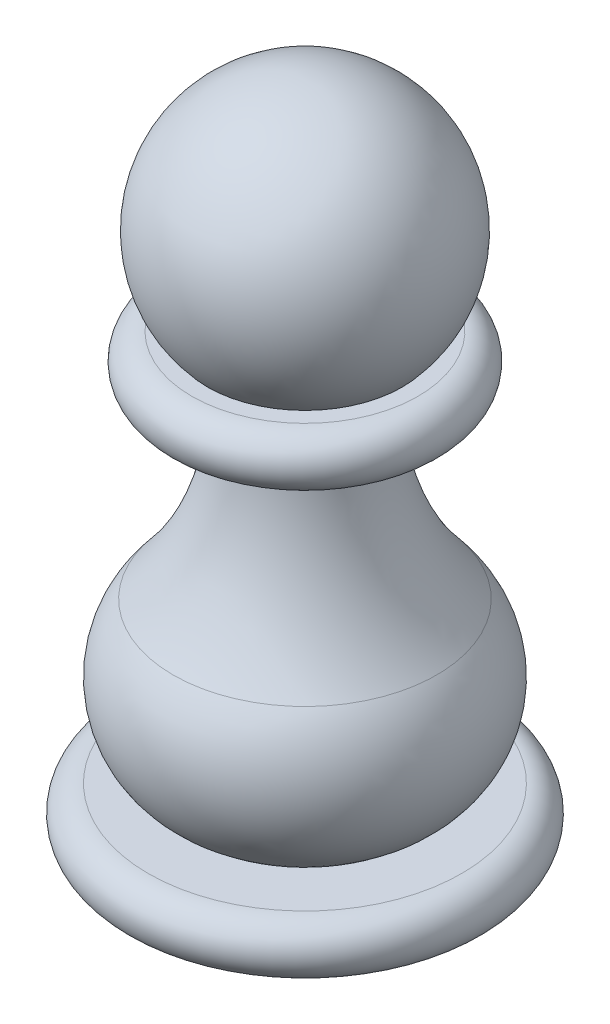
ISO-10303-21;
HEADER;
FILE_DESCRIPTION(('STEP AP214'),'2;1');
FILE_NAME('part.step','',(''),(''),'','','');
FILE_SCHEMA(('AUTOMOTIVE_DESIGN { 1 0 10303 214 1 1 1 1 }'));
ENDSEC;
DATA;
#1=APPLICATION_CONTEXT('core data for automotive mechanical design processes');
#2=APPLICATION_PROTOCOL_DEFINITION('international standard','automotive_design',2000,#1);
#3=PRODUCT_CONTEXT('',#1,'mechanical');
#4=PRODUCT('Part','Part','',(#3));
#5=PRODUCT_RELATED_PRODUCT_CATEGORY('part','',(#4));
#6=PRODUCT_DEFINITION_FORMATION('','',#4);
#7=PRODUCT_DEFINITION_CONTEXT('part definition',#1,'design');
#8=PRODUCT_DEFINITION('design','',#6,#7);
#9=PRODUCT_DEFINITION_SHAPE('','',#8);
#10=(LENGTH_UNIT() NAMED_UNIT(*) SI_UNIT(.MILLI.,.METRE.));
#11=(NAMED_UNIT(*) PLANE_ANGLE_UNIT() SI_UNIT($,.RADIAN.));
#12=(NAMED_UNIT(*) SI_UNIT($,.STERADIAN.) SOLID_ANGLE_UNIT());
#13=UNCERTAINTY_MEASURE_WITH_UNIT(LENGTH_MEASURE(1.E-05),#10,'distance_accuracy_value','');
#14=(GEOMETRIC_REPRESENTATION_CONTEXT(3) GLOBAL_UNCERTAINTY_ASSIGNED_CONTEXT((#13)) GLOBAL_UNIT_ASSIGNED_CONTEXT((#10,
#11,#12)) REPRESENTATION_CONTEXT('',''));
#15=CARTESIAN_POINT('',(0.,0.,0.));
#16=DIRECTION('',(0.,0.,1.));
#17=DIRECTION('',(1.,0.,0.));
#18=AXIS2_PLACEMENT_3D('',#15,#16,#17);
#19=CARTESIAN_POINT('',(0.,-7.5,0.));
#20=DIRECTION('',(0.,1.,0.));
#21=DIRECTION('',(1.,0.,0.));
#22=AXIS2_PLACEMENT_3D('',#19,#20,#21);
#23=SPHERICAL_SURFACE('',#22,7.5);
#24=CARTESIAN_POINT('',(0.,-12.5,0.));
#25=DIRECTION('',(0.,1.,0.));
#26=DIRECTION('',(0.,0.,1.));
#27=AXIS2_PLACEMENT_3D('',#24,#25,#26);
#28=CIRCLE('',#27,5.59016994374947);
#29=CARTESIAN_POINT('',(0.,-12.5,5.59016994374947));
#30=VERTEX_POINT('',#29);
#31=EDGE_CURVE('E11',#30,#30,#28,.T.);
#32=ORIENTED_EDGE('',*,*,#31,.T.);
#33=EDGE_LOOP('',(#32));
#34=FACE_BOUND('',#33,.T.);
#35=ADVANCED_FACE('F45',(#34),#23,.T.);
#36=CARTESIAN_POINT('',(0.,-12.5,0.));
#37=DIRECTION('',(0.,1.,0.));
#38=DIRECTION('',(0.,0.,1.));
#39=AXIS2_PLACEMENT_3D('',#36,#37,#38);
#40=PLANE('',#39);
#41=CARTESIAN_POINT('',(0.,-12.5,0.));
#42=DIRECTION('',(0.,1.,0.));
#43=DIRECTION('',(0.,0.,1.));
#44=AXIS2_PLACEMENT_3D('',#41,#42,#43);
#45=CIRCLE('',#44,6.5);
#46=CARTESIAN_POINT('',(0.,-12.5,6.5));
#47=VERTEX_POINT('',#46);
#48=EDGE_CURVE('E47',#47,#47,#45,.T.);
#49=ORIENTED_EDGE('',*,*,#48,.T.);
#50=EDGE_LOOP('',(#49));
#51=FACE_BOUND('',#50,.T.);
#52=ORIENTED_EDGE('',*,*,#31,.F.);
#53=EDGE_LOOP('',(#52));
#54=FACE_BOUND('',#53,.T.);
#55=ADVANCED_FACE('F87',(#51,#54),#40,.T.);
#56=CARTESIAN_POINT('',(0.,-14.,0.));
#57=DIRECTION('',(0.,1.,0.));
#58=DIRECTION('',(0.,0.,1.));
#59=AXIS2_PLACEMENT_3D('',#56,#57,#58);
#60=TOROIDAL_SURFACE('',#59,6.5,1.5);
#61=CARTESIAN_POINT('',(0.,-15.5,0.));
#62=DIRECTION('',(0.,1.,0.));
#63=DIRECTION('',(0.,0.,1.));
#64=AXIS2_PLACEMENT_3D('',#61,#62,#63);
#65=CIRCLE('',#64,6.5);
#66=CARTESIAN_POINT('',(0.,-15.5,6.5));
#67=VERTEX_POINT('',#66);
#68=EDGE_CURVE('E84',#67,#67,#65,.T.);
#69=ORIENTED_EDGE('',*,*,#68,.T.);
#70=EDGE_LOOP('',(#69));
#71=FACE_BOUND('',#70,.T.);
#72=ORIENTED_EDGE('',*,*,#48,.F.);
#73=EDGE_LOOP('',(#72));
#74=FACE_BOUND('',#73,.T.);
#75=ADVANCED_FACE('F89',(#71,#74),#60,.T.);
#76=CARTESIAN_POINT('',(0.,-15.5,0.));
#77=DIRECTION('',(0.,1.,0.));
#78=DIRECTION('',(0.,0.,1.));
#79=AXIS2_PLACEMENT_3D('',#76,#77,#78);
#80=PLANE('',#79);
#81=ORIENTED_EDGE('',*,*,#68,.F.);
#82=EDGE_LOOP('',(#81));
#83=FACE_BOUND('',#82,.T.);
#84=CARTESIAN_POINT('',(0.,-15.5,0.));
#85=DIRECTION('',(0.,1.,0.));
#86=DIRECTION('',(0.,0.,1.));
#87=AXIS2_PLACEMENT_3D('',#84,#85,#86);
#88=CIRCLE('',#87,4.);
#89=CARTESIAN_POINT('',(0.,-15.5,4.));
#90=VERTEX_POINT('',#89);
#91=EDGE_CURVE('E76',#90,#90,#88,.T.);
#92=ORIENTED_EDGE('',*,*,#91,.T.);
#93=EDGE_LOOP('',(#92));
#94=FACE_BOUND('',#93,.T.);
#95=ADVANCED_FACE('F95',(#83,#94),#80,.F.);
#96=CARTESIAN_POINT('',(0.,0.,0.));
#97=DIRECTION('',(0.,1.,0.));
#98=DIRECTION('',(0.,0.,1.));
#99=AXIS2_PLACEMENT_3D('',#96,#97,#98);
#100=CYLINDRICAL_SURFACE('',#99,4.);
#101=CARTESIAN_POINT('',(0.,-16.1175255425094,0.));
#102=DIRECTION('',(0.,1.,0.));
#103=DIRECTION('',(0.,0.,1.));
#104=AXIS2_PLACEMENT_3D('',#101,#102,#103);
#105=CIRCLE('',#104,4.);
#106=CARTESIAN_POINT('',(0.,-16.1175255425094,4.));
#107=VERTEX_POINT('',#106);
#108=EDGE_CURVE('E77',#107,#107,#105,.T.);
#109=ORIENTED_EDGE('',*,*,#108,.T.);
#110=EDGE_LOOP('',(#109));
#111=FACE_BOUND('',#110,.T.);
#112=ORIENTED_EDGE('',*,*,#91,.F.);
#113=EDGE_LOOP('',(#112));
#114=FACE_BOUND('',#113,.T.);
#115=ADVANCED_FACE('F97',(#111,#114),#100,.T.);
#116=CARTESIAN_POINT('',(0.,-16.1175255425094,0.));
#117=DIRECTION('',(0.,1.,0.));
#118=DIRECTION('',(0.,0.,1.));
#119=AXIS2_PLACEMENT_3D('',#116,#117,#118);
#120=TOROIDAL_SURFACE('',#119,19.,15.);
#121=CARTESIAN_POINT('',(0.,-25.8328616201775,0.));
#122=DIRECTION('',(0.,1.,0.));
#123=DIRECTION('',(0.,0.,1.));
#124=AXIS2_PLACEMENT_3D('',#121,#122,#123);
#125=CIRCLE('',#124,7.57142857142858);
#126=CARTESIAN_POINT('',(0.,-25.8328616201775,7.57142857142858));
#127=VERTEX_POINT('',#126);
#128=EDGE_CURVE('E71',#127,#127,#125,.T.);
#129=ORIENTED_EDGE('',*,*,#128,.T.);
#130=EDGE_LOOP('',(#129));
#131=FACE_BOUND('',#130,.T.);
#132=ORIENTED_EDGE('',*,*,#108,.F.);
#133=EDGE_LOOP('',(#132));
#134=FACE_BOUND('',#133,.T.);
#135=ADVANCED_FACE('F135',(#131,#134),#120,.F.);
#136=CARTESIAN_POINT('',(0.,-29.7189960512448,0.));
#137=DIRECTION('',(0.,1.,0.));
#138=DIRECTION('',(0.,0.,1.));
#139=AXIS2_PLACEMENT_3D('',#136,#137,#138);
#140=DEGENERATE_TOROIDAL_SURFACE('',#139,3.,6.00000000000001,.T.);
#141=CARTESIAN_POINT('',(0.,-35.,0.));
#142=DIRECTION('',(0.,1.,0.));
#143=DIRECTION('',(0.,0.,1.));
#144=AXIS2_PLACEMENT_3D('',#141,#142,#143);
#145=CIRCLE('',#144,5.84798126630638);
#146=CARTESIAN_POINT('',(0.,-35.,5.84798126630638));
#147=VERTEX_POINT('',#146);
#148=EDGE_CURVE('E68',#147,#147,#145,.T.);
#149=ORIENTED_EDGE('',*,*,#148,.T.);
#150=EDGE_LOOP('',(#149));
#151=FACE_BOUND('',#150,.T.);
#152=ORIENTED_EDGE('',*,*,#128,.F.);
#153=EDGE_LOOP('',(#152));
#154=FACE_BOUND('',#153,.T.);
#155=ADVANCED_FACE('F142',(#151,#154),#140,.T.);
#156=CARTESIAN_POINT('',(0.,-35.,0.));
#157=DIRECTION('',(0.,1.,0.));
#158=DIRECTION('',(0.,0.,1.));
#159=AXIS2_PLACEMENT_3D('',#156,#157,#158);
#160=PLANE('',#159);
#161=CARTESIAN_POINT('',(0.,-35.,0.));
#162=DIRECTION('',(0.,1.,0.));
#163=DIRECTION('',(0.,0.,1.));
#164=AXIS2_PLACEMENT_3D('',#161,#162,#163);
#165=CIRCLE('',#164,8.99999999999998);
#166=CARTESIAN_POINT('',(0.,-35.,8.99999999999998));
#167=VERTEX_POINT('',#166);
#168=EDGE_CURVE('E63',#167,#167,#165,.T.);
#169=ORIENTED_EDGE('',*,*,#168,.T.);
#170=EDGE_LOOP('',(#169));
#171=FACE_BOUND('',#170,.T.);
#172=ORIENTED_EDGE('',*,*,#148,.F.);
#173=EDGE_LOOP('',(#172));
#174=FACE_BOUND('',#173,.T.);
#175=ADVANCED_FACE('F155',(#171,#174),#160,.T.);
#176=CARTESIAN_POINT('',(0.,-36.5,0.));
#177=DIRECTION('',(0.,1.,0.));
#178=DIRECTION('',(0.,0.,1.));
#179=AXIS2_PLACEMENT_3D('',#176,#177,#178);
#180=TOROIDAL_SURFACE('',#179,9.00000000000001,1.5);
#181=CARTESIAN_POINT('',(0.,-38.,0.));
#182=DIRECTION('',(0.,1.,0.));
#183=DIRECTION('',(0.,0.,1.));
#184=AXIS2_PLACEMENT_3D('',#181,#182,#183);
#185=CIRCLE('',#184,8.99999999999998);
#186=CARTESIAN_POINT('',(0.,-38.,8.99999999999998));
#187=VERTEX_POINT('',#186);
#188=EDGE_CURVE('E65',#187,#187,#185,.T.);
#189=ORIENTED_EDGE('',*,*,#188,.T.);
#190=EDGE_LOOP('',(#189));
#191=FACE_BOUND('',#190,.T.);
#192=ORIENTED_EDGE('',*,*,#168,.F.);
#193=EDGE_LOOP('',(#192));
#194=FACE_BOUND('',#193,.T.);
#195=ADVANCED_FACE('F165',(#191,#194),#180,.T.);
#196=CARTESIAN_POINT('',(0.,-38.,0.));
#197=DIRECTION('',(0.,1.,0.));
#198=DIRECTION('',(0.,0.,1.));
#199=AXIS2_PLACEMENT_3D('',#196,#197,#198);
#200=PLANE('',#199);
#201=ORIENTED_EDGE('',*,*,#188,.F.);
#202=EDGE_LOOP('',(#201));
#203=FACE_BOUND('',#202,.T.);
#204=ADVANCED_FACE('F175',(#203),#200,.F.);
#205=CLOSED_SHELL('',(#35,#55,#75,#95,#115,#135,#155,#175,#195,#204));
#206=CARTESIAN_POINT('',(0.,-35.,0.));
#207=DIRECTION('',(0.,1.,0.));
#208=DIRECTION('',(0.,0.,1.));
#209=AXIS2_PLACEMENT_3D('',#206,#207,#208);
#210=CIRCLE('',#209,0.152018733693616);
#211=CARTESIAN_POINT('',(0.,-35.,0.152018733693616));
#212=VERTEX_POINT('',#211);
#213=EDGE_CURVE('E58',#212,#212,#210,.T.);
#214=ORIENTED_EDGE('',*,*,#213,.T.);
#215=EDGE_LOOP('',(#214));
#216=FACE_BOUND('',#215,.T.);
#217=ADVANCED_FACE('F54',(#216),#160,.T.);
#218=CARTESIAN_POINT('',(0.,-29.7189960512448,3.));
#219=DIRECTION('',(-1.,0.,0.));
#220=DIRECTION('',(0.,0.,1.));
#221=AXIS2_PLACEMENT_3D('',#218,#219,#220);
#222=CIRCLE('',#221,6.00000000000001);
#223=TRIMMED_CURVE('',#222,(PARAMETER_VALUE(-2.09439510239319)),
(PARAMETER_VALUE(2.09439510239319)),.T.,.PARAMETER.);
#224=CARTESIAN_POINT('',(0.,-29.7189960512448,0.));
#225=DIRECTION('',(0.,1.,0.));
#226=AXIS1_PLACEMENT('',#224,#225);
#227=SURFACE_OF_REVOLUTION('',#223,#226);
#228=CARTESIAN_POINT('',(0.,-34.9151484739514,0.));
#229=VERTEX_POINT('',#228);
#230=VERTEX_LOOP('',#229);
#231=FACE_BOUND('',#230,.T.);
#232=ORIENTED_EDGE('',*,*,#213,.F.);
#233=EDGE_LOOP('',(#232));
#234=FACE_BOUND('',#233,.T.);
#235=ADVANCED_FACE('F55',(#231,#234),#227,.T.);
#236=CLOSED_SHELL('',(#217,#235));
#237=ORIENTED_CLOSED_SHELL('',*,#236,.T.);
#238=BREP_WITH_VOIDS('B2',#205,(#237));
#239=ADVANCED_BREP_SHAPE_REPRESENTATION('',(#18,#238),#14);
#240=SHAPE_DEFINITION_REPRESENTATION(#9,#239);
ENDSEC;
END-ISO-10303-21;
